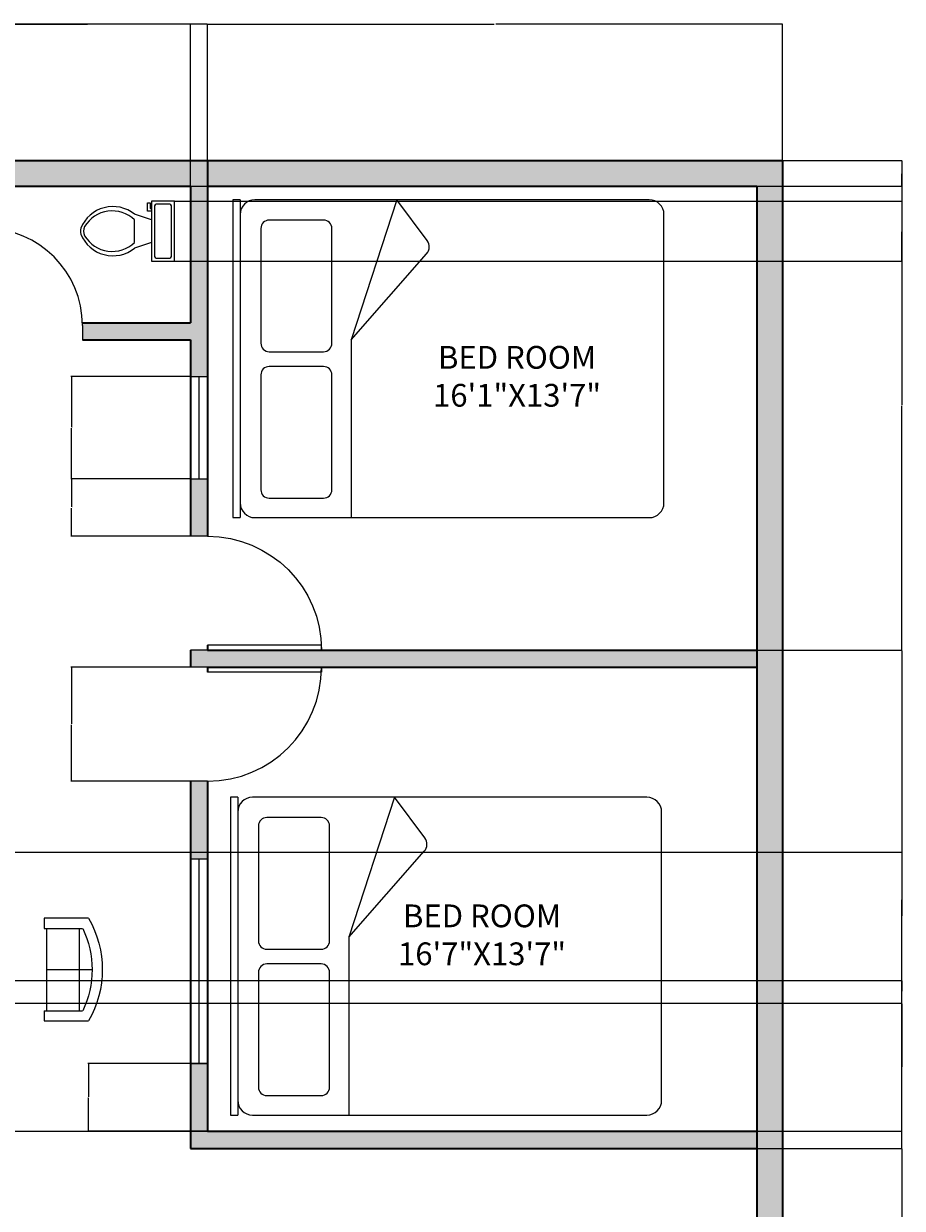
# Model space of a CAD drawing. Units: inches. Extents: x -89 to 661, y -827 to 77.
# Tile 5 of 5: x 353 to 661, y -339 to 77. Entities that reach past the tile are written whole.
import ezdxf

# ---------------------------------------------------------------- set-up
doc = ezdxf.new("R2010")
doc.units = ezdxf.units.IN
doc.header["$MEASUREMENT"] = 0
for name, color, linetype, lineweight in [('A-ANNO-DIMS', 2, 'Continuous', 18), ('A-AREA-IDEN', 7, 'Continuous', 18), ('A-FLOR-FIXT', 9, 'Continuous', 18), ('A-FURN', 34, 'Continuous', 18), ('A-GLAZ', 5, 'Continuous', 18), ('A-WALL', 7, 'Continuous', 35), ('A-WALL-PATT', 30, 'Continuous', 13), ('DOOR', 5, 'Continuous', 25)]:
    doc.layers.add(name, color=color, linetype=linetype, lineweight=lineweight)
doc.styles.get("Standard").update_dxf_attribs({"font": 'arial.ttf'})
doc.dimstyles.get("Standard").update_dxf_attribs({"dimtxt": 0.18, "dimasz": 0.18, "dimexe": 0.18, "dimexo": 0.0625, "dimgap": 0.09, "dimtad": 0, "dimtih": 1, "dimtoh": 1, "dimdec": 4, "dimzin": 0, "dimdsep": 46, "dimtxsty": 'Standard', "dimcen": 0.09, "dimadec": 0, "dimazin": 0, "dimtfac": 1, "dimtdec": 4, "dimtofl": 0, "dimtmove": 0, "dimatfit": 3, "dimfxl": 1, "dimtolj": 1, "dimtzin": 0, "dimarcsym": 0})

# ---------------------------------------------------------------- blocks, each defined once
blk = doc.blocks.new('*U7')
for p, q in [((0, 0), (0, -6)), ((40, 0), (40, -6))]:
    blk.add_line(p, q)
blk.add_lwpolyline([(0, 0), (0, 40), (1.75, 40), (1.75, 0)], close=True)
blk.add_arc((0, 0), 40, 0, 90)
blk = doc.blocks.new('A$C164346CA')
for p, q in [((0, 2.035), (0, 2)), ((1.5, 2.035), (0, 2.035)), ((1.5, 2), (1.5, 2.035)), ((1.5, 2), (0, 2)), ((0, 1.93), (0, 0.07)), ((0.6731, 1.9024), (0.1319, 1.9024)), ((1.364, 1.9024), (0.8228, 1.9024)), ((1.5, 0.07), (1.5, 1.93)), ((0.0919, 1.8624), (0.0919, 1.6069)), ((0.7131, 1.6069), (0.7131, 1.8624)), ((0.7828, 1.8624), (0.7828, 1.6069)), ((1.404, 1.6069), (1.404, 1.8624)), ((0.1319, 1.5669), (0.6731, 1.5669)), ((0.8228, 1.5669), (1.364, 1.5669)), ((0.8395, 1.4761), (0, 1.4761)), ((0.8395, 1.4761), (1.2448, 1.12)), ((1.5, 1.2611), (0.8395, 1.4761)), ((1.3077, 1.1175), (1.5, 1.2611)), ((0.07, 0), (1.43, 0))]:
    blk.add_line(p, q)
for centre, radius, start, end in [((0.07, 1.93), 0.07, 90, 180), ((1.43, 1.93), 0.07, 0, 90), ((0.1319, 1.8624), 0.04, 90, 180), ((0.6731, 1.8624), 0.04, 0, 90), ((0.8228, 1.8624), 0.04, 90, 180), ((1.364, 1.8624), 0.04, 0, 90), ((0.1319, 1.6069), 0.04, 180, 270), ((0.6731, 1.6069), 0.04, 270, 0), ((0.8228, 1.6069), 0.04, 180, 270), ((1.364, 1.6069), 0.04, 270, 0), ((1.2778, 1.1575), 0.05, 228.6958, 306.7579), ((0.07, 0.07), 0.07, 180, 270), ((1.43, 0.07), 0.07, 270, 0)]:
    blk.add_arc(centre, radius, start, end)
blk = doc.blocks.new('A$C01575E38')
for p, q in [((0.75, 0.039), (0.75, 0.7)), ((0.75, 0.039), (0.75, 0.7)), ((0, 0), (0, 0.65)), ((0, 0), (0, 0.65)), ((0.15, 0), (0.15, 0.563)), ((0.15, 0), (0.15, 0.563)), ((1.35, 0), (1.35, 0.563)), ((1.35, 0), (1.35, 0.563)), ((1.5, 0.65), (1.5, 0)), ((1.5, 0.65), (1.5, 0)), ((0.15, 0.515), (1.35, 0.515)), ((0.15, 0.515), (1.35, 0.515)), ((0.15, 0), (0, 0)), ((0.15, 0), (0, 0)), ((0.15, 0.039), (1.35, 0.039)), ((0.15, 0.039), (1.35, 0.039)), ((1.5, 0), (1.35, 0)), ((1.5, 0), (1.35, 0))]:
    blk.add_line(p, q)
for centre, radius, start, end in [((0.75, -0.656), 1.506, 60.1372, 119.8628), ((0.75, -0.656), 1.506, 60.1372, 119.8628), ((0.75, -0.685), 1.385, 64.3208, 115.6792), ((0.75, -0.685), 1.385, 64.3208, 115.6792)]:
    blk.add_arc(centre, radius, start, end)
blk = doc.blocks.new('*U15')
for p, q in [((9.5, -6), (9.5, -2)), ((-8, -8.5), (-8, -8)), ((-7, -8), (-7, -9.5)), ((-4, -8), (-6, -14)), ((4, -8), (6, -14)), ((-10, -8.5), (-8, -8.5)), ((-10, -9.5), (-10, -8.5)), ((-7, -9.5), (-10, -9.5)), ((4, -14), (-4, -14))]:
    blk.add_line(p, q)
blk.add_lwpolyline([(10.5, -8), (10.5, 0), (-10.5, 0), (-10.5, -8)], close=True)
for points in [[(-9.5, -2), (-9.5, -6)], [(8.5, -1), (-8.5, -1)], [(-8.5, -7), (8.5, -7)]]:
    blk.add_lwpolyline(points)
for centre, radius, start, end in [((-8.62, -1.88), 0.884, 81.8699, 188.1301), ((8.62, -1.88), 0.884, 351.8699, 98.1301), ((-8.62, -6.12), 0.884, 171.8699, 278.1301), ((8.62, -6.12), 0.884, 261.8699, 8.1301), ((3.52, -21.58), 12.17, 141.4691, 247.9714), ((4.2, -21.82), 11.33, 136.3677, 238.9468), ((-3.52, -21.58), 12.17, 292.0284, 38.5307), ((-4.2, -21.82), 11.33, 301.053, 43.6321), ((0, -27.88), 4, 245.7318, 294.2682), ((0, -29), 4, 254.8605, 285.1395)]:
    blk.add_arc(centre, radius, start, end)
blk = doc.blocks.new('WIN-72-NOM')
for p, q in [((0, 6), (0, 0)), ((0, 6), (71.86, 6)), ((71.86, 6), (71.86, 0)), ((0, 3), (71.86, 3)), ((0, 0), (71.86, 0))]:
    blk.add_line(p, q)
blk = doc.blocks.new('*D34')
at = {"layer": 'A-ANNO-DIMS', "color": 0, "lineweight": -2, "transparency": 16777216}
for p, q in [((417.19, 29.12), (417.19, 77.13)), ((417.37, 76.95), (517.9, 76.95)), ((619.01, 76.95), (518.48, 76.95)), ((619.19, 29.12), (619.19, 77.13))]:
    blk.add_line(p, q, dxfattribs=at)
at = {"layer": 'A-ANNO-DIMS', "color": 0, "transparency": 16777216}
for points in [[(417.37, 76.98), (417.37, 76.92), (417.19, 76.95)], [(619.01, 76.98), (619.01, 76.92), (619.19, 76.95)]]:
    blk.add_solid(points, dxfattribs=at)
at = {"layer": 'Defpoints', "color": 0, "transparency": 16777216}
for p in [(619.19, 76.95), (417.19, 29.06), (619.19, 29.06)]:
    blk.add_point(p, dxfattribs=at)
at = {"layer": 'A-ANNO-DIMS', "color": 0, "transparency": 16777216, "insert": (518.19, 76.95), "char_height": 0.18, "attachment_point": 5}
blk.add_mtext('\\A1;202', dxfattribs=at)
blk = doc.blocks.new('*D35')
at = {"layer": 'A-ANNO-DIMS', "color": 0, "lineweight": -2, "transparency": 16777216}
for p, q in [((619.25, 29.06), (661.23, 29.06)), ((661.05, 28.88), (661.05, -56.76)), ((661.05, -142.76), (661.05, -57.12)), ((610.25, -142.94), (661.23, -142.94))]:
    blk.add_line(p, q, dxfattribs=at)
at = {"layer": 'A-ANNO-DIMS', "color": 0, "transparency": 16777216}
for points in [[(661.02, 28.88), (661.08, 28.88), (661.05, 29.06)], [(661.02, -142.76), (661.08, -142.76), (661.05, -142.94)]]:
    blk.add_solid(points, dxfattribs=at)
at = {"layer": 'Defpoints', "color": 0, "transparency": 16777216}
for p in [(619.19, 29.06), (661.05, 29.06), (610.19, -142.94)]:
    blk.add_point(p, dxfattribs=at)
at = {"layer": 'A-ANNO-DIMS', "color": 0, "transparency": 16777216, "insert": (661.05, -56.94), "char_height": 0.18, "attachment_point": 5}
blk.add_mtext('\\A1;172', dxfattribs=at)
blk = doc.blocks.new('*D36')
at = {"layer": 'A-ANNO-DIMS', "color": 0, "lineweight": -2, "transparency": 16777216}
for p, q in [((610.25, -142.94), (661.23, -142.94)), ((661.05, -143.12), (661.05, -230.26)), ((661.05, -317.76), (661.05, -230.62)), ((610.25, -317.94), (661.23, -317.94))]:
    blk.add_line(p, q, dxfattribs=at)
at = {"layer": 'A-ANNO-DIMS', "color": 0, "transparency": 16777216}
for points in [[(661.02, -143.12), (661.08, -143.12), (661.05, -142.94)], [(661.02, -317.76), (661.08, -317.76), (661.05, -317.94)]]:
    blk.add_solid(points, dxfattribs=at)
at = {"layer": 'Defpoints', "color": 0, "transparency": 16777216}
for p in [(610.19, -142.94), (661.05, -142.94), (610.19, -317.94)]:
    blk.add_point(p, dxfattribs=at)
at = {"layer": 'A-ANNO-DIMS', "color": 0, "transparency": 16777216, "insert": (661.05, -230.44), "char_height": 0.18, "attachment_point": 5}
blk.add_mtext('\\A1;175', dxfattribs=at)
blk = doc.blocks.new('*D37')
at = {"layer": 'A-ANNO-DIMS', "color": 0, "lineweight": -2, "transparency": 16777216}
for p, q in [((610.25, -317.94), (661.23, -317.94)), ((661.05, -318.12), (661.05, -371.76)), ((661.05, -425.76), (661.05, -372.12)), ((610.25, -425.94), (661.23, -425.94))]:
    blk.add_line(p, q, dxfattribs=at)
at = {"layer": 'A-ANNO-DIMS', "color": 0, "transparency": 16777216}
for points in [[(661.02, -318.12), (661.08, -318.12), (661.05, -317.94)], [(661.02, -425.76), (661.08, -425.76), (661.05, -425.94)]]:
    blk.add_solid(points, dxfattribs=at)
at = {"layer": 'Defpoints', "color": 0, "transparency": 16777216}
for p in [(610.19, -317.94), (661.05, -317.94), (610.19, -425.94)]:
    blk.add_point(p, dxfattribs=at)
at = {"layer": 'A-ANNO-DIMS', "color": 0, "transparency": 16777216, "insert": (661.05, -371.94), "char_height": 0.18, "attachment_point": 5}
blk.add_mtext('\\A1;108', dxfattribs=at)
blk = doc.blocks.new('*D41')
at = {"layer": 'A-ANNO-DIMS', "color": 0, "lineweight": -2, "transparency": 16777216}
for p, q in [((255.19, 29.12), (255.19, 77.13)), ((255.37, 76.95), (335.91, 76.95)), ((417.01, 76.95), (336.47, 76.95)), ((417.19, 29.12), (417.19, 77.13))]:
    blk.add_line(p, q, dxfattribs=at)
at = {"layer": 'A-ANNO-DIMS', "color": 0, "transparency": 16777216}
for points in [[(255.37, 76.98), (255.37, 76.92), (255.19, 76.95)], [(417.01, 76.98), (417.01, 76.92), (417.19, 76.95)]]:
    blk.add_solid(points, dxfattribs=at)
at = {"layer": 'Defpoints', "color": 0, "transparency": 16777216}
for p in [(417.19, 76.95), (255.19, 29.06), (417.19, 29.06)]:
    blk.add_point(p, dxfattribs=at)
at = {"layer": 'A-ANNO-DIMS', "color": 0, "transparency": 16777216, "insert": (336.19, 76.95), "char_height": 0.18, "attachment_point": 5}
blk.add_mtext('\\A1;162', dxfattribs=at)
blk = doc.blocks.new('*D45')
at = {"layer": 'A-ANNO-DIMS', "color": 0, "lineweight": -2, "transparency": 16777216}
for p, q in [((339.19, 20.12), (339.19, 77.13)), ((339.37, 76.95), (374.97, 76.95)), ((411.01, 76.95), (375.4, 76.95)), ((411.19, 20.12), (411.19, 77.13))]:
    blk.add_line(p, q, dxfattribs=at)
at = {"layer": 'A-ANNO-DIMS', "color": 0, "transparency": 16777216}
for points in [[(339.37, 76.98), (339.37, 76.92), (339.19, 76.95)], [(411.01, 76.98), (411.01, 76.92), (411.19, 76.95)]]:
    blk.add_solid(points, dxfattribs=at)
at = {"layer": 'Defpoints', "color": 0, "transparency": 16777216}
for p in [(411.19, 76.95), (339.19, 20.06), (411.19, 20.06)]:
    blk.add_point(p, dxfattribs=at)
at = {"layer": 'A-ANNO-DIMS', "color": 0, "transparency": 16777216, "insert": (375.19, 76.95), "char_height": 0.18, "attachment_point": 5}
blk.add_mtext('\\A1;72', dxfattribs=at)
blk = doc.blocks.new('*D47')
at = {"layer": 'A-ANNO-DIMS', "color": 0, "lineweight": -2, "transparency": 16777216}
for p, q in [((417.25, 29.06), (661.23, 29.06)), ((661.05, 28.88), (661.05, 24.74)), ((661.05, 20.24), (661.05, 24.38)), ((411.25, 20.06), (661.23, 20.06))]:
    blk.add_line(p, q, dxfattribs=at)
at = {"layer": 'A-ANNO-DIMS', "color": 0, "transparency": 16777216}
for points in [[(661.02, 28.88), (661.08, 28.88), (661.05, 29.06)], [(661.02, 20.24), (661.08, 20.24), (661.05, 20.06)]]:
    blk.add_solid(points, dxfattribs=at)
at = {"layer": 'Defpoints', "color": 0, "transparency": 16777216}
for p in [(417.19, 29.06), (661.05, 29.06), (411.19, 20.06)]:
    blk.add_point(p, dxfattribs=at)
at = {"layer": 'A-ANNO-DIMS', "color": 0, "transparency": 16777216, "insert": (661.05, 24.56), "char_height": 0.18, "attachment_point": 5}
blk.add_mtext('\\A1;9', dxfattribs=at)
blk = doc.blocks.new('*D49')
at = {"layer": 'A-ANNO-DIMS', "color": 0, "lineweight": -2, "transparency": 16777216}
for p, q in [((405.58, 14.75), (661.23, 14.75)), ((661.05, 14.57), (661.05, 4.43)), ((661.05, -6.07), (661.05, 4.07)), ((405.58, -6.25), (661.23, -6.25))]:
    blk.add_line(p, q, dxfattribs=at)
at = {"layer": 'A-ANNO-DIMS', "color": 0, "transparency": 16777216}
for points in [[(661.02, 14.57), (661.08, 14.57), (661.05, 14.75)], [(661.02, -6.07), (661.08, -6.07), (661.05, -6.25)]]:
    blk.add_solid(points, dxfattribs=at)
at = {"layer": 'Defpoints', "color": 0, "transparency": 16777216}
for p in [(405.51, 14.75), (661.05, 14.75), (405.51, -6.25)]:
    blk.add_point(p, dxfattribs=at)
at = {"layer": 'A-ANNO-DIMS', "color": 0, "transparency": 16777216, "insert": (661.05, 4.25), "char_height": 0.18, "attachment_point": 5}
blk.add_mtext('\\A1;21', dxfattribs=at)
blk = doc.blocks.new('*D50')
at = {"layer": 'A-ANNO-DIMS', "color": 0, "lineweight": -2, "transparency": 16777216}
for p, q in [((212.9, -213.94), (661.23, -213.94)), ((661.05, -214.12), (661.05, -236.26)), ((661.05, -258.76), (661.05, -236.62)), ((212.9, -258.94), (661.23, -258.94))]:
    blk.add_line(p, q, dxfattribs=at)
at = {"layer": 'A-ANNO-DIMS', "color": 0, "transparency": 16777216}
for points in [[(661.02, -214.12), (661.08, -214.12), (661.05, -213.94)], [(661.02, -258.76), (661.08, -258.76), (661.05, -258.94)]]:
    blk.add_solid(points, dxfattribs=at)
at = {"layer": 'Defpoints', "color": 0, "transparency": 16777216}
for p in [(212.84, -213.94), (661.05, -213.94), (212.84, -258.94)]:
    blk.add_point(p, dxfattribs=at)
at = {"layer": 'A-ANNO-DIMS', "color": 0, "transparency": 16777216, "insert": (661.05, -236.44), "char_height": 0.18, "attachment_point": 5}
blk.add_mtext('\\A1;45', dxfattribs=at)
blk = doc.blocks.new('*D51')
at = {"layer": 'A-ANNO-DIMS', "color": 0, "lineweight": -2, "transparency": 16777216}
for p, q in [((188.9, -266.94), (661.23, -266.94)), ((661.05, -267.12), (661.05, -289.26)), ((661.05, -311.76), (661.05, -289.62)), ((188.9, -311.94), (661.23, -311.94))]:
    blk.add_line(p, q, dxfattribs=at)
at = {"layer": 'A-ANNO-DIMS', "color": 0, "transparency": 16777216}
for points in [[(661.02, -267.12), (661.08, -267.12), (661.05, -266.94)], [(661.02, -311.76), (661.08, -311.76), (661.05, -311.94)]]:
    blk.add_solid(points, dxfattribs=at)
at = {"layer": 'Defpoints', "color": 0, "transparency": 16777216}
for p in [(188.84, -266.94), (661.05, -266.94), (188.84, -311.94)]:
    blk.add_point(p, dxfattribs=at)
at = {"layer": 'A-ANNO-DIMS', "color": 0, "transparency": 16777216, "insert": (661.05, -289.44), "char_height": 0.18, "attachment_point": 5}
blk.add_mtext('\\A1;45', dxfattribs=at)
blk = doc.blocks.new('*D52')
at = {"layer": 'A-ANNO-DIMS', "color": 0, "lineweight": -2, "transparency": 16777216}
for p, q in [((212.9, -258.94), (661.23, -258.94)), ((661.05, -259.12), (661.05, -262.76)), ((661.05, -266.76), (661.05, -263.12)), ((212.9, -266.94), (661.23, -266.94))]:
    blk.add_line(p, q, dxfattribs=at)
at = {"layer": 'A-ANNO-DIMS', "color": 0, "transparency": 16777216}
for points in [[(661.02, -259.12), (661.08, -259.12), (661.05, -258.94)], [(661.02, -266.76), (661.08, -266.76), (661.05, -266.94)]]:
    blk.add_solid(points, dxfattribs=at)
at = {"layer": 'Defpoints', "color": 0, "transparency": 16777216}
for p in [(212.84, -258.94), (661.05, -258.94), (212.84, -266.94)]:
    blk.add_point(p, dxfattribs=at)
at = {"layer": 'A-ANNO-DIMS', "color": 0, "transparency": 16777216, "insert": (661.05, -262.94), "char_height": 0.18, "attachment_point": 5}
blk.add_mtext('\\A1;8', dxfattribs=at)
blk = doc.blocks.new('*D65')
at = {"layer": 'A-ANNO-DIMS', "color": 0, "lineweight": -2, "transparency": 16777216}
for p, q in [((411.12, -46.77), (369.15, -46.77)), ((369.33, -46.95), (369.33, -64.55)), ((369.33, -82.52), (369.33, -64.92)), ((411.12, -82.7), (369.15, -82.7))]:
    blk.add_line(p, q, dxfattribs=at)
at = {"layer": 'A-ANNO-DIMS', "color": 0, "transparency": 16777216}
for points in [[(369.3, -46.95), (369.36, -46.95), (369.33, -46.77)], [(369.3, -82.52), (369.36, -82.52), (369.33, -82.7)]]:
    blk.add_solid(points, dxfattribs=at)
at = {"layer": 'Defpoints', "color": 0, "transparency": 16777216}
for p in [(369.33, -46.77), (411.19, -46.77), (411.19, -82.7)]:
    blk.add_point(p, dxfattribs=at)
at = {"layer": 'A-ANNO-DIMS', "color": 0, "transparency": 16777216, "insert": (369.33, -64.74), "char_height": 0.18, "attachment_point": 5}
blk.add_mtext('\\A1;35.93', dxfattribs=at)
blk = doc.blocks.new('*D71')
at = {"layer": 'A-ANNO-DIMS', "color": 0, "lineweight": -2, "transparency": 16777216}
for p, q in [((411.12, -82.7), (369.15, -82.7)), ((369.33, -82.88), (369.33, -92.64)), ((369.33, -102.76), (369.33, -93)), ((411.12, -102.94), (369.15, -102.94))]:
    blk.add_line(p, q, dxfattribs=at)
at = {"layer": 'A-ANNO-DIMS', "color": 0, "transparency": 16777216}
for points in [[(369.3, -82.88), (369.36, -82.88), (369.33, -82.7)], [(369.3, -102.76), (369.36, -102.76), (369.33, -102.94)]]:
    blk.add_solid(points, dxfattribs=at)
at = {"layer": 'Defpoints', "color": 0, "transparency": 16777216}
for p in [(369.33, -82.7), (411.19, -82.7), (411.19, -102.94)]:
    blk.add_point(p, dxfattribs=at)
at = {"layer": 'A-ANNO-DIMS', "color": 0, "transparency": 16777216, "insert": (369.33, -92.82), "char_height": 0.18, "attachment_point": 5}
blk.add_mtext('\\A1;20.24', dxfattribs=at)
blk = doc.blocks.new('*D72')
at = {"layer": 'A-ANNO-DIMS', "color": 0, "lineweight": -2, "transparency": 16777216}
for p, q in [((417.12, -288.11), (375.15, -288.11)), ((375.33, -288.29), (375.33, -299.84)), ((375.33, -311.76), (375.33, -300.21)), ((417.12, -311.94), (375.15, -311.94))]:
    blk.add_line(p, q, dxfattribs=at)
at = {"layer": 'A-ANNO-DIMS', "color": 0, "transparency": 16777216}
for points in [[(375.3, -288.29), (375.36, -288.29), (375.33, -288.11)], [(375.3, -311.76), (375.36, -311.76), (375.33, -311.94)]]:
    blk.add_solid(points, dxfattribs=at)
at = {"layer": 'Defpoints', "color": 0, "transparency": 16777216}
for p in [(375.33, -288.11), (417.19, -288.11), (417.19, -311.94)]:
    blk.add_point(p, dxfattribs=at)
at = {"layer": 'A-ANNO-DIMS', "color": 0, "transparency": 16777216, "insert": (375.33, -300.03), "char_height": 0.18, "attachment_point": 5}
blk.add_mtext('\\A1;23.83', dxfattribs=at)
blk = doc.blocks.new('*D76')
at = {"layer": 'A-ANNO-DIMS', "color": 0, "lineweight": -2, "transparency": 16777216}
for p, q in [((411.12, -148.94), (369.15, -148.94)), ((369.33, -149.12), (369.33, -168.76)), ((369.33, -188.76), (369.33, -169.12)), ((411.12, -188.94), (369.15, -188.94))]:
    blk.add_line(p, q, dxfattribs=at)
at = {"layer": 'A-ANNO-DIMS', "color": 0, "transparency": 16777216}
for points in [[(369.3, -149.12), (369.36, -149.12), (369.33, -148.94)], [(369.3, -188.76), (369.36, -188.76), (369.33, -188.94)]]:
    blk.add_solid(points, dxfattribs=at)
at = {"layer": 'Defpoints', "color": 0, "transparency": 16777216}
for p in [(369.33, -148.94), (411.19, -148.94), (411.19, -188.94)]:
    blk.add_point(p, dxfattribs=at)
at = {"layer": 'A-ANNO-DIMS', "color": 0, "transparency": 16777216, "insert": (369.33, -168.94), "char_height": 0.18, "attachment_point": 5}
blk.add_mtext('\\A1;40', dxfattribs=at)

msp = doc.modelspace()

# ---------------------------------------------------------------- hatches: boundary and pattern name
at = {"layer": 'A-WALL-PATT'}
h = msp.add_hatch(color=256, dxfattribs=at)
h.dxf.hatch_style = 1
h.paths.add_polyline_path([(610.186, -311.94), (417.186, -311.94), (417.186, -288.111), (411.186, -288.111), (411.186, -317.94), (610.186, -317.94)])
h.paths.add_polyline_path([(417.186, -188.94), (411.186, -188.94), (411.186, -216.247), (417.186, -216.247)])
h.paths.add_polyline_path([(610.186, -142.94), (417.186, -142.94), (411.186, -142.94), (411.186, -148.94), (417.186, -148.94), (457.186, -148.94), (610.186, -148.94)])
h.paths.add_polyline_path([(417.186, -82.701), (411.186, -82.701), (411.186, -102.94), (417.186, -102.94)])
h.paths.add_polyline_path([(261.186, -124.327), (255.186, -124.327), (255.186, -167.94), (261.186, -167.94)])
h.paths.add_polyline_path([(261.186, 20.06), (333.186, 20.06), (333.186, -33.94), (339.186, -33.94), (339.186, -28.84), (339.186, 5.16), (339.186, 20.06), (411.186, 20.06), (411.186, -27.94), (373.174, -27.94, -0.0066185), (373.186, -28.84), (373.186, -33.94), (411.186, -33.94), (411.186, -46.769), (417.186, -46.769), (417.186, 29.06), (255.186, 29.06), (255.186, -52.464), (261.186, -52.464), (261.186, -33.94), (299.186, -33.94), (299.186, -28.84, -0.0066185), (299.198, -27.94), (261.186, -27.94)])
h.paths.add_polyline_path([(261.186, -207.94), (255.186, -207.94), (215.186, -207.94), (7.186, -207.94), (7.186, -213.94), (261.186, -213.94)])
h.paths.add_polyline_path([(212.837, -311.94), (7.186, -311.94), (7.186, -317.94), (212.837, -317.94)])
h = msp.add_hatch(color=256, dxfattribs=at)
h.dxf.hatch_style = 1
h.paths.add_polyline_path([(619.186, 29.06), (417.186, 29.06), (417.186, 20.06), (610.186, 20.06), (610.186, -142.94), (610.186, -311.94), (610.186, -419.94), (516.186, -419.94), (516.186, -425.94), (610.186, -425.94), (610.186, -527.94), (610.186, -533.94), (619.186, -533.94)])

# ---------------------------------------------------------------- linework, layer by layer
at = {"layer": 'A-GLAZ'}
for p, q in [((411.186, -46.769), (417.186, -46.769)), ((411.186, -82.701), (411.186, -46.769)), ((414.186, -82.701), (414.186, -46.769)), ((417.186, -82.701), (417.186, -46.769)), ((411.186, -82.701), (417.186, -82.701))]:
    msp.add_line(p, q, dxfattribs=at)
at = {"layer": 'A-WALL'}
for p, q in [((-1.814, 29.06), (619.186, 29.06)), ((417.186, 29.06), (417.186, -102.94)), ((619.186, 29.06), (619.186, -782.94)), ((339.186, 20.06), (411.186, 20.06)), ((411.186, 20.06), (411.186, -27.94)), ((417.186, 20.06), (610.186, 20.06)), ((610.186, 20.06), (610.186, -142.94)), ((373.174, -27.94), (411.186, -27.94)), ((373.186, -33.94), (411.186, -33.94)), ((411.186, -33.94), (411.186, -102.94)), ((417.186, -141.19), (417.186, -142.94)), ((411.186, -142.94), (411.186, -148.94)), ((417.186, -142.94), (610.186, -142.94)), ((610.186, -142.94), (610.186, -311.94)), ((417.186, -148.94), (610.186, -148.94)), ((417.186, -148.94), (417.186, -150.69)), ((411.186, -188.94), (411.186, -317.94)), ((417.186, -188.94), (417.186, -311.94)), ((417.186, -311.94), (610.186, -311.94)), ((610.186, -311.94), (610.186, -419.94)), ((411.186, -317.94), (610.186, -317.94))]:
    msp.add_line(p, q, dxfattribs=at)

# ---------------------------------------------------------------- block references
at = {"layer": 'A-FLOR-FIXT', "rotation": 270}
msp.add_blockref('*U15', (405.514, 4.25), dxfattribs=at)
at = {"layer": 'A-FURN'}
for name, p, xscale, yscale, zscale, rotation in [('A$C164346CA', (577.526, -96.383), 74.45384008536578, 74.45384008536578, 74.45384008536578, 90), ('A$C164346CA', (576.698, -306.264), 74.45384008536578, 74.45384008536578, 74.45384008536578, 90), ('A$C01575E38', (359.751, -273.197), -24.05223591321487, 24.05223591321487, 24.05223591321487, 270)]:
    msp.add_blockref(name, p, dxfattribs=dict(at, xscale=xscale, yscale=yscale, zscale=zscale, rotation=rotation))
at = {"layer": 'A-GLAZ', "rotation": 89.99999999999991}
msp.add_blockref('WIN-72-NOM', (417.186, -288.111), dxfattribs=at)
at = {"layer": 'DOOR', "xscale": 0.85, "yscale": 0.85, "zscale": 0.85}
msp.add_blockref('*U7', (339.186, -28.84), dxfattribs=at)
at = {"layer": 'DOOR', "xscale": -1, "rotation": 270}
msp.add_blockref('*U7', (417.186, -142.94), dxfattribs=at)
at = {"layer": 'DOOR', "rotation": 270}
msp.add_blockref('*U7', (417.186, -148.94), dxfattribs=at)

# ---------------------------------------------------------------- texts
at = {"layer": 'A-AREA-IDEN', "char_height": 8, "attachment_point": 1}
for s, width, insert in [('\\pxqc;BED ROOM\\P16\'1"X13\'7"', 130.31124, (460.751, -36.072)), ('\\pxqc;BED ROOM\\P16\'7"X13\'7"', 80.04851, (473.58, -232.271))]:
    msp.add_mtext_dynamic_manual_height_columns(s, width=width, gutter_width=1, heights=[0], dxfattribs=dict(at, insert=insert))

# ---------------------------------------------------------------- dimensions: what is measured, and where the dimension line sits
at = {"layer": 'A-ANNO-DIMS'}
for base, p1, p2, picture, middle in [((417.186, 76.952), (255.186, 29.06), (417.186, 29.06), '*D41', (336.186, 76.952)), ((411.186, 76.952), (339.186, 20.06), (411.186, 20.06), '*D45', (375.186, 76.952)), ((619.186, 76.952), (417.186, 29.06), (619.186, 29.06), '*D34', (518.186, 76.952))]:
    dim = msp.add_linear_dim(base=base, p1=p1, p2=p2, dimstyle='Standard', override={"dimdec": 0, "dimlfac": 1, "dimrnd": 0, "dimzin": 0, "dimdsep": 46, "dimlunit": 2}, dxfattribs=at)
    dim.commit()
    dim.dimension.update_dxf_attribs({"geometry": picture, "text_midpoint": middle})
for base, p1, p2, override, picture, middle in [((661.046, 29.06), (411.186, 20.06), (417.186, 29.06), {"dimdec": 0, "dimlfac": 1, "dimrnd": 0, "dimzin": 0, "dimdsep": 46, "dimlunit": 2}, '*D47', (661.046, 24.56)), ((661.046, 29.06), (610.186, -142.94), (619.186, 29.06), {"dimdec": 0, "dimlfac": 1, "dimrnd": 0, "dimzin": 0, "dimdsep": 46, "dimlunit": 2}, '*D35', (661.046, -56.94)), ((661.046, 14.75), (405.514, -6.25), (405.514, 14.75), {"dimdec": 0, "dimlfac": 1, "dimrnd": 0, "dimzin": 0, "dimdsep": 46, "dimlunit": 2}, '*D49', (661.046, 4.25)), ((369.326, -46.769), (411.186, -82.701), (411.186, -46.769), {"dimdec": 2, "dimlfac": 1, "dimrnd": 0, "dimzin": 0, "dimdsep": 46, "dimlunit": 2}, '*D65', (369.326, -64.735)), ((369.326, -82.701), (411.186, -102.94), (411.186, -82.701), {"dimdec": 2, "dimlfac": 1, "dimrnd": 0, "dimzin": 0, "dimdsep": 46, "dimlunit": 2}, '*D71', (369.326, -92.82)), ((661.046, -142.94), (610.186, -317.94), (610.186, -142.94), {"dimdec": 0, "dimlfac": 1, "dimrnd": 0, "dimzin": 0, "dimdsep": 46, "dimlunit": 2}, '*D36', (661.046, -230.44)), ((369.326, -148.94), (411.186, -188.94), (411.186, -148.94), {"dimdec": 0, "dimlfac": 1, "dimrnd": 0, "dimzin": 0, "dimdsep": 46, "dimlunit": 2}, '*D76', (369.326, -168.94)), ((661.046, -213.94), (212.837, -258.94), (212.837, -213.94), {"dimdec": 0, "dimlfac": 1, "dimrnd": 0, "dimzin": 0, "dimdsep": 46, "dimlunit": 2}, '*D50', (661.046, -236.44)), ((661.046, -258.94), (212.837, -266.94), (212.837, -258.94), {"dimdec": 0, "dimlfac": 1, "dimrnd": 0, "dimzin": 0, "dimdsep": 46, "dimlunit": 2}, '*D52', (661.046, -262.94)), ((661.046, -266.94), (188.837, -311.94), (188.837, -266.94), {"dimdec": 0, "dimlfac": 1, "dimrnd": 0, "dimzin": 0, "dimdsep": 46, "dimlunit": 2}, '*D51', (661.046, -289.44)), ((375.326, -288.111), (417.186, -311.94), (417.186, -288.111), {"dimdec": 2, "dimlfac": 1, "dimrnd": 0, "dimzin": 0, "dimdsep": 46, "dimlunit": 2}, '*D72', (375.326, -300.025)), ((661.046, -317.94), (610.186, -425.94), (610.186, -317.94), {"dimdec": 0, "dimlfac": 1, "dimrnd": 0, "dimzin": 0, "dimdsep": 46, "dimlunit": 2}, '*D37', (661.046, -371.94))]:
    dim = msp.add_linear_dim(base=base, p1=p1, p2=p2, angle=90, dimstyle='Standard', override=override, dxfattribs=at)
    dim.commit()
    dim.dimension.update_dxf_attribs({"geometry": picture, "text_midpoint": middle})

doc.saveas('drawing.dxf')
